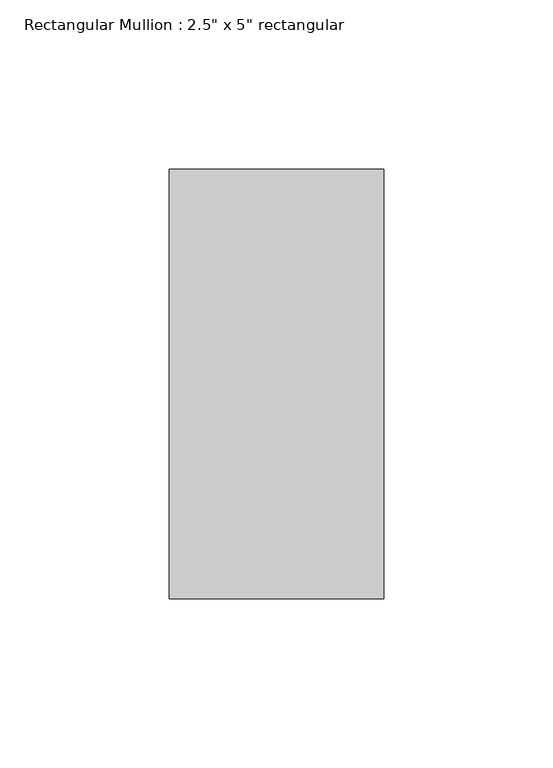
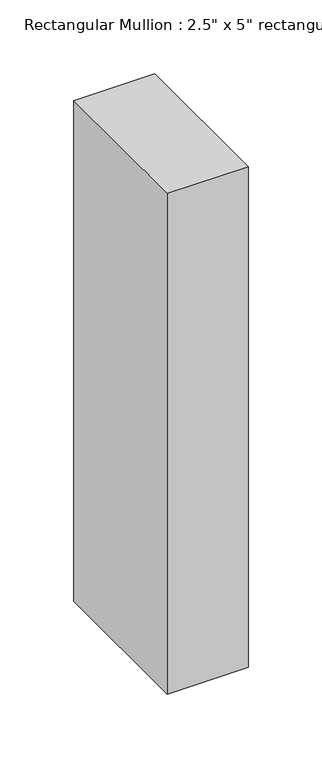
"""IFC4 building model written with IfcOpenShell, lengths in millimetres: member geometry."""

from ifc_helpers import new_model, si_unit, frame, origin, place, context, project, spatial, polyline, outline, extrude, source, transform, mapped, element, save


def member_cc20b924(model_context):
    return source(origin(), model_context, "Body", "SweptSolid", [
        extrude(outline(polyline([(0.0, 63.5), (0.0, -63.5), (-63.5, -63.5), (-63.5, 63.5), (0.0, 63.5)])), frame((0.0, 0.0, -414.8666667), z_axis=(0.0, 0.0, 1.0), x_axis=(1.0, 0.0, 0.0)), (0.0, 0.0, 1.0), 414.8666667),
    ])


if __name__ == "__main__":
    model = new_model("IFC4")
    model_context = context("Model", 3, world=origin())
    ifc_project = project(units=[si_unit("LENGTHUNIT", "METRE", prefix="MILLI")], contexts=[model_context])
    site = spatial("IfcSite", under=ifc_project)
    building = spatial("IfcBuilding", under=site)
    placement = place(None, origin())
    member_shape = member_cc20b924(model_context)
    element("IfcMember", 1, ObjectType="Rectangular Mullion : 2.5\" x 5\" rectangular", at=placement, inside=building, context=model_context, shape_type="MappedRepresentation", body=[
        mapped(member_shape, transform((0.0, 0.0, 0.0), x_axis=(1.0, 0.0, 0.0), y_axis=(0.0, 1.0, 0.0), z_axis=(0.0, 0.0, 1.0))),
    ])
    save(model, "model.ifc")

# Revit data of these elements
# Type "Rectangular Mullion : 2.5\" x 5\" rectangular"
#   built-in parameter 1007304 = 0.416667 (stored number, unit not read)
#   built-in parameter 1007301 = 0.104167 (stored number, unit not read)
#   built-in parameter 1007300 = 0.104167 (stored number, unit not read)
# Element 1 (IfcMember, "Rectangular Mullion : 2.5\" x 5\" rectangular")
#   Materials on its faces: "Aluminum"
# Materials
#   "Aluminum": class "Metal", colour RGB 247 247 247, transparency 0, Description = "Aluminum 6061", Cost = 0
